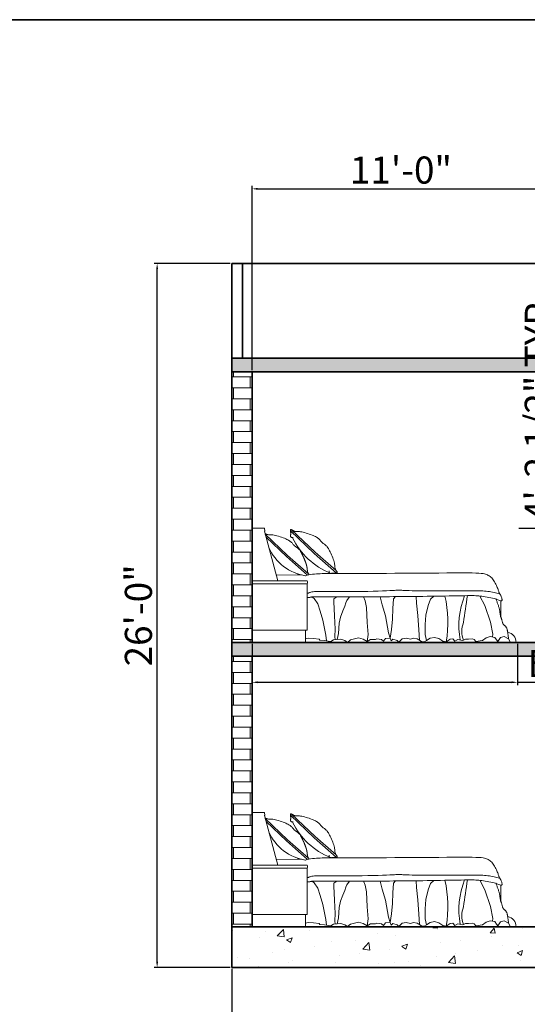
# Model space of a CAD drawing. Units: inches. Extents: x 2142 to 3604, y 1690 to 2981.
# Tile 7 of 9: x 2829 to 3054, y 2545 to 2981. Entities that reach past the tile are written whole.
import ezdxf

# ---------------------------------------------------------------- set-up
doc = ezdxf.new("R2010")
doc.units = ezdxf.units.IN
for name, color, linetype, lineweight in [('A-ANNO-DIMS', 2, 'Continuous', 18), ('A-ANNO-TTLB', 7, 'Continuous', 35), ('A-FLOR-PATT', 8, 'Continuous', 13), ('A-FURN', 8, 'Continuous', 18), ('A-SECT', 7, 'Continuous', 35), ('A-WALL-PATT', 8, 'Continuous', 13)]:
    doc.layers.add(name, color=color, linetype=linetype, lineweight=lineweight)
doc.styles.get("Standard").update_dxf_attribs({"font": 'arial.ttf'})
doc.dimstyles.new('ISO-25', dxfattribs={"dimtxt": 12, "dimasz": 2.5, "dimexe": 1.25, "dimexo": 0.625, "dimtad": 1, "dimdec": 0, "dimlunit": 3, "dimtxsty": 'Standard', "dimcen": 2.5, "dimadec": 0, "dimazin": 0, "dimtfac": 1, "dimtdec": 0, "dimtmove": 0, "dimatfit": 3, "dimfxl": 1, "dimarcsym": 0})

# ---------------------------------------------------------------- blocks, each defined once
blk = doc.blocks.new('A$C08BC4B9A')
for p, q in [((0, 924.5), (0.5, 925)), ((0, 0), (0, 924.5)), ((95, 925), (0.5, 925)), ((101.1, 921.9), (105, 907.4)), ((101.4, 901.2), (208.9, 500)), ((106.6, 881.7), (106.8, 881.6)), ((106.8, 881.6), (109.7, 879.8)), ((109.7, 879.8), (112.8, 878.1)), ((112.8, 878.1), (116.3, 876.5)), ((311.4, 909.3), (311.5, 910.8)), ((311.5, 907.6), (311.4, 909.3)), ((311.5, 910.8), (311.7, 912.1)), ((311.7, 905.6), (311.5, 907.6)), ((311.7, 912.1), (312.1, 913.2)), ((312, 903.5), (311.7, 905.6)), ((502.9, 721.7), (311.9, 904.5)), ((312.3, 901.1), (312, 903.5)), ((312.1, 913.2), (312.7, 914.1)), ((312.6, 898.6), (312.3, 901.1)), ((312.9, 895.9), (312.6, 898.6)), ((312.7, 914.1), (313.6, 914.7)), ((313.1, 892.9), (312.9, 895.9)), ((313.3, 889.8), (313.1, 892.9)), ((313.4, 886.5), (313.3, 889.8)), ((313.3, 875.5), (313.4, 879.4)), ((313.4, 883), (313.4, 886.5)), ((313.4, 879.4), (313.4, 883)), ((313.6, 914.7), (314.7, 915)), ((314.7, 915), (316, 915.1)), ((316, 915.1), (317.6, 914.9)), ((317.6, 914.9), (319.3, 914.5)), ((319.3, 914.5), (321.1, 913.7)), ((511.6, 731.1), (320.5, 913.9)), ((321.1, 913.7), (323.2, 912.6)), ((323.2, 912.6), (325.4, 911.2)), ((325.4, 911.2), (327.8, 909.6)), ((327.8, 909.6), (330.4, 907.8)), ((330.4, 907.8), (333.3, 906.1)), ((333.3, 906.1), (336.4, 904.3)), ((336.4, 904.3), (339.9, 902.7)), ((339.9, 902.7), (343.7, 901.4)), ((343.7, 901.4), (347.9, 900.4)), ((347.9, 900.4), (352.5, 899.8)), ((352.5, 899.8), (357.6, 899.5)), ((357.6, 899.5), (363.2, 899.4)), ((363.2, 899.4), (369.6, 899.2)), ((369.6, 899.2), (376.7, 898.9)), ((376.7, 898.9), (384.6, 898.3)), ((384.6, 898.3), (393.4, 897.3)), ((393.4, 897.3), (403.3, 895.7)), ((403.3, 895.7), (414.2, 893.3)), ((414.2, 893.3), (425.9, 890.4)), ((425.9, 890.4), (438.1, 886.9)), ((438.1, 886.9), (450.5, 883.1)), ((450.5, 883.1), (462.9, 878.9)), ((462.9, 878.9), (474.9, 874.6)), ((288, 704.9), (107.8, 877.3)), ((279.2, 695.5), (114.2, 853.4)), ((116.3, 876.5), (120.1, 875.2)), ((120.1, 875.2), (124.3, 874.2)), ((124.3, 874.2), (128.9, 873.6)), ((128.9, 873.6), (134, 873.3)), ((134, 873.3), (139.6, 873.2)), ((139.6, 873.2), (146, 873)), ((146, 873), (153.1, 872.7)), ((153.1, 872.7), (161, 872.1)), ((161, 872.1), (169.8, 871.1)), ((169.8, 871.1), (179.7, 869.5)), ((179.7, 869.5), (190.6, 867.1)), ((190.6, 867.1), (202.3, 864.2)), ((202.3, 864.2), (214.5, 860.7)), ((214.5, 860.7), (226.9, 856.8)), ((226.9, 856.8), (239.3, 852.7)), ((239.3, 852.7), (251.3, 848.4)), ((251.3, 848.4), (262.7, 844)), ((262.7, 844), (273.2, 839.6)), ((273.2, 839.6), (282.5, 835.5)), ((282.5, 835.5), (290.7, 831.4)), ((290.7, 831.4), (298, 827.4)), ((298, 827.4), (304.4, 823.4)), ((304.4, 823.4), (310.1, 819.5)), ((310.1, 819.5), (315.2, 815.4)), ((312.7, 863.2), (312.8, 867.3)), ((313.1, 859.2), (312.7, 863.2)), ((312.8, 867.3), (313, 871.5)), ((313, 871.5), (313.3, 875.5)), ((314.3, 855.7), (313.1, 859.2)), ((316.7, 852.8), (314.3, 855.7)), ((315.2, 815.4), (319.8, 811.3)), ((320.4, 850.8), (316.7, 852.8)), ((319.8, 811.3), (324.1, 807)), ((325.8, 849.7), (320.4, 850.8)), ((324.1, 807), (328.1, 802.5)), ((333.2, 849.9), (325.8, 849.7)), ((328.1, 802.5), (332, 797.9)), ((332, 797.9), (335.8, 793.2)), ((474.9, 874.6), (486.3, 870.2)), ((486.3, 870.2), (496.8, 865.9)), ((496.8, 865.9), (506.1, 861.7)), ((506.1, 861.7), (514.3, 857.6)), ((514.3, 857.6), (521.6, 853.6)), ((521.6, 853.6), (528, 849.7)), ((528, 849.7), (533.7, 845.7)), ((533.7, 845.7), (538.8, 841.7)), ((538.8, 841.7), (543.4, 837.5)), ((543.4, 837.5), (547.7, 833.2)), ((547.7, 833.2), (551.7, 828.7)), ((551.7, 828.7), (555.6, 824.1)), ((555.6, 824.1), (559.4, 819.4)), ((559.4, 819.4), (563.3, 814.6)), ((563.3, 814.6), (567.7, 810.4)), ((572.2, 806.3), (567.7, 810.4)), ((577.3, 802.8), (572.2, 806.3)), ((582.3, 799.4), (577.3, 802.8)), ((587.2, 795.8), (582.3, 799.4)), ((335.8, 793.2), (339.7, 788.4)), ((339.7, 788.4), (344.1, 784.1)), ((344.2, 784), (344.1, 784.1)), ((344.5, 783.8), (344.2, 784)), ((344.9, 783.4), (344.5, 783.8)), ((345.5, 782.9), (344.9, 783.4)), ((346.1, 782.3), (345.5, 782.9)), ((346.8, 781.7), (346.1, 782.3)), ((347.6, 781.1), (346.8, 781.7)), ((348.3, 780.5), (347.6, 781.1)), ((349.1, 779.9), (348.3, 780.5)), ((349.8, 779.4), (349.1, 779.9)), ((350.5, 778.9), (349.8, 779.4)), ((351.1, 778.4), (350.5, 778.9)), ((351.8, 777.9), (351.1, 778.4)), ((352.4, 777.5), (351.8, 777.9)), ((353.1, 777), (352.4, 777.5)), ((353.7, 776.6), (353.1, 777)), ((354.3, 776.2), (353.7, 776.6)), ((354.9, 775.7), (354.3, 776.2)), ((355.6, 775.3), (354.9, 775.7)), ((356.2, 774.9), (355.6, 775.3)), ((356.8, 774.4), (356.2, 774.9)), ((357.4, 774), (356.8, 774.4)), ((358.1, 773.6), (357.4, 774)), ((358.7, 773.1), (358.1, 773.6)), ((359.3, 772.7), (358.7, 773.1)), ((359.9, 772.3), (359.3, 772.7)), ((360.5, 771.8), (359.9, 772.3)), ((361.2, 771.4), (360.5, 771.8)), ((361.8, 770.9), (361.2, 771.4)), ((362.4, 770.5), (361.8, 770.9)), ((363, 770), (362.4, 770.5)), ((363.6, 769.6), (363, 770)), ((364.2, 769.1), (363.6, 769.6)), ((364.8, 768.7), (364.2, 769.1)), ((365.4, 768.2), (364.8, 768.7)), ((366, 767.8), (365.4, 768.2)), ((366.6, 767.3), (366, 767.8)), ((367.2, 766.8), (366.6, 767.3)), ((367.8, 766.4), (367.2, 766.8)), ((368.3, 765.9), (367.8, 766.4)), ((368.9, 765.4), (368.3, 765.9)), ((369.5, 764.9), (368.9, 765.4)), ((370.1, 764.4), (369.5, 764.9)), ((370.7, 763.9), (370.1, 764.4)), ((371.2, 763.5), (370.7, 763.9)), ((371.8, 763), (371.2, 763.5)), ((372.4, 762.4), (371.8, 763)), ((373, 761.9), (372.4, 762.4)), ((373.5, 761.4), (373, 761.9)), ((374.1, 760.9), (373.5, 761.4)), ((374.7, 760.4), (374.1, 760.9)), ((375.2, 759.8), (374.7, 760.4)), ((375.8, 759.3), (375.2, 759.8)), ((376.3, 758.7), (375.8, 759.3)), ((376.9, 758.2), (376.3, 758.7)), ((377.4, 757.6), (376.9, 758.2)), ((378, 757), (377.4, 757.6)), ((378.6, 756.5), (378, 757)), ((379.2, 755.8), (378.6, 756.5)), ((379.8, 755.2), (379.2, 755.8)), ((380.5, 754.5), (379.8, 755.2)), ((381.3, 753.8), (380.5, 754.5)), ((382.2, 753.1), (381.3, 753.8)), ((383.2, 752.3), (382.2, 753.1)), ((384.2, 751.4), (383.2, 752.3)), ((385.4, 750.5), (384.2, 751.4)), ((386.6, 749.6), (385.4, 750.5)), ((387.8, 748.7), (386.6, 749.6)), ((388.9, 747.8), (387.8, 748.7)), ((389.9, 746.9), (388.9, 747.8)), ((390.8, 746), (389.9, 746.9)), ((391.4, 745.3), (390.8, 746)), ((391.9, 744.6), (391.4, 745.3)), ((392.1, 744), (391.9, 744.6)), ((392, 741.9), (392.1, 742.4)), ((392, 741.3), (392, 741.9)), ((392, 740.8), (392, 741.3)), ((392.1, 740.1), (392, 740.8)), ((392.2, 743.4), (392.1, 744)), ((392.1, 742.4), (392.2, 742.9)), ((392.4, 739.4), (392.1, 740.1)), ((392.2, 742.9), (392.2, 743.4)), ((392.7, 738.6), (392.4, 739.4)), ((393.1, 737.8), (392.7, 738.6)), ((393.6, 737), (393.1, 737.8)), ((394.1, 736.1), (393.6, 737)), ((394.7, 735.2), (394.1, 736.1)), ((395.2, 734.3), (394.7, 735.2)), ((395.8, 733.4), (395.2, 734.3)), ((396.4, 732.4), (395.8, 733.4)), ((397, 731.5), (396.4, 732.4)), ((397.6, 730.5), (397, 731.5)), ((398.2, 729.5), (397.6, 730.5)), ((398.7, 728.5), (398.2, 729.5)), ((399.3, 727.4), (398.7, 728.5)), ((399.9, 726.4), (399.3, 727.4)), ((400.5, 725.3), (399.9, 726.4)), ((401.1, 724.3), (400.5, 725.3)), ((401.7, 723.2), (401.1, 724.3)), ((402.4, 722), (401.7, 723.2)), ((403, 720.9), (402.4, 722)), ((403.6, 719.8), (403, 720.9)), ((404.2, 718.6), (403.6, 719.8)), ((404.8, 717.4), (404.2, 718.6)), ((685.7, 562.3), (502.9, 721.7)), ((681.3, 583.2), (511.6, 731.1)), ((592, 792.2), (587.2, 795.8)), ((596.6, 788.2), (592, 792.2)), ((601.1, 783.9), (596.6, 788.2)), ((605.5, 779.1), (601.1, 783.9)), ((609.9, 773.7), (605.5, 779.1)), ((614.3, 767.6), (609.9, 773.7)), ((618.8, 760.7), (614.3, 767.6)), ((623.5, 752.8), (618.8, 760.7)), ((628.4, 743.8), (623.5, 752.8)), ((633.5, 733.7), (628.4, 743.8)), ((638.7, 722.7), (633.5, 733.7)), ((643.9, 711), (638.7, 722.7)), ((450.1, 546.6), (279.2, 695.5)), ((457.7, 557), (288, 704.9)), ((405.4, 716.2), (404.8, 717.4)), ((406.1, 715), (405.4, 716.2)), ((406.7, 713.8), (406.1, 715)), ((407.3, 712.5), (406.7, 713.8)), ((408, 711.2), (407.3, 712.5)), ((408.6, 710), (408, 711.2)), ((409.3, 708.7), (408.6, 710)), ((409.9, 707.3), (409.3, 708.7)), ((410.6, 706), (409.9, 707.3)), ((411.2, 704.7), (410.6, 706)), ((411.9, 703.3), (411.2, 704.7)), ((412.5, 701.9), (411.9, 703.3)), ((413.2, 700.6), (412.5, 701.9)), ((413.8, 699.2), (413.2, 700.6)), ((414.5, 697.8), (413.8, 699.2)), ((415.1, 696.4), (414.5, 697.8)), ((415.8, 694.9), (415.1, 696.4)), ((416.4, 693.5), (415.8, 694.9)), ((417.1, 692.1), (416.4, 693.5)), ((417.7, 690.6), (417.1, 692.1)), ((418.4, 689.2), (417.7, 690.6)), ((419, 687.7), (418.4, 689.2)), ((419.7, 686.2), (419, 687.7)), ((420.3, 684.7), (419.7, 686.2)), ((421, 683.3), (420.3, 684.7)), ((421.6, 681.8), (421, 683.3)), ((422.2, 680.3), (421.6, 681.8)), ((422.9, 678.8), (422.2, 680.3)), ((423.5, 677.3), (422.9, 678.8)), ((424.1, 675.8), (423.5, 677.3)), ((424.7, 674.3), (424.1, 675.8)), ((425.4, 672.8), (424.7, 674.3)), ((426, 671.3), (425.4, 672.8)), ((426.6, 669.7), (426, 671.3)), ((427.2, 668.2), (426.6, 669.7)), ((427.8, 666.7), (427.2, 668.2)), ((428.4, 665.2), (427.8, 666.7)), ((429, 663.7), (428.4, 665.2)), ((429.6, 662.2), (429, 663.7)), ((430.1, 660.7), (429.6, 662.2)), ((430.7, 659.2), (430.1, 660.7)), ((431.3, 657.7), (430.7, 659.2)), ((431.8, 656.2), (431.3, 657.7)), ((432.4, 654.7), (431.8, 656.2)), ((432.9, 653.2), (432.4, 654.7)), ((433.4, 651.8), (432.9, 653.2)), ((434, 650.3), (433.4, 651.8)), ((434.5, 648.8), (434, 650.3)), ((435, 647.4), (434.5, 648.8)), ((435.5, 645.9), (435, 647.4)), ((436, 644.5), (435.5, 645.9)), ((436.5, 643.1), (436, 644.5)), ((436.9, 641.7), (436.5, 643.1)), ((437.4, 640.2), (436.9, 641.7)), ((437.9, 638.8), (437.4, 640.2)), ((438.3, 637.5), (437.9, 638.8)), ((649, 699), (643.9, 711)), ((653.8, 686.9), (649, 699)), ((658.2, 675), (653.8, 686.9)), ((662, 663.6), (658.2, 675)), ((665.2, 652.9), (662, 663.6)), ((667.5, 643.2), (665.2, 652.9)), ((669.2, 634.4), (667.5, 643.2)), ((438.7, 636.1), (438.3, 637.5)), ((439.1, 634.7), (438.7, 636.1)), ((439.6, 633.4), (439.1, 634.7)), ((440, 632), (439.6, 633.4)), ((440.3, 630.7), (440, 632)), ((440.7, 629.4), (440.3, 630.7)), ((441.1, 628.1), (440.7, 629.4)), ((441.4, 626.8), (441.1, 628.1)), ((441.8, 625.5), (441.4, 626.8)), ((442.1, 624.3), (441.8, 625.5)), ((442.4, 623.1), (442.1, 624.3)), ((442.7, 621.8), (442.4, 623.1)), ((443, 620.6), (442.7, 621.8)), ((443.3, 619.4), (443, 620.6)), ((443.6, 618.3), (443.3, 619.4)), ((443.8, 617.1), (443.6, 618.3)), ((444.1, 616), (443.8, 617.1)), ((444.3, 614.8), (444.1, 616)), ((444.5, 613.7), (444.3, 614.8)), ((444.7, 612.6), (444.5, 613.7)), ((445, 611.5), (444.7, 612.6)), ((445.2, 610.5), (445, 611.5)), ((445.4, 609.4), (445.2, 610.5)), ((445.5, 608.4), (445.4, 609.4)), ((445.7, 607.3), (445.5, 608.4)), ((445.9, 606.3), (445.7, 607.3)), ((446, 605.3), (445.9, 606.3)), ((446.2, 604.3), (446, 605.3)), ((446.4, 603.3), (446.2, 604.3)), ((446.5, 602.4), (446.4, 603.3)), ((446.6, 601.4), (446.5, 602.4)), ((446.8, 600.5), (446.6, 601.4)), ((446.9, 599.6), (446.8, 600.5)), ((447, 598.6), (446.9, 599.6)), ((447.1, 597.7), (447, 598.6)), ((447.2, 596.9), (447.1, 597.7)), ((447.3, 596), (447.2, 596.9)), ((447.4, 595.1), (447.3, 596)), ((447.5, 594.3), (447.4, 595.1)), ((447.6, 593.4), (447.5, 594.3)), ((447.7, 592.6), (447.6, 593.4)), ((447.8, 591.8), (447.7, 592.6)), ((447.9, 591), (447.8, 591.8)), ((448, 590.2), (447.9, 591)), ((448, 589.4), (448, 590.2)), ((448.1, 588.6), (448, 589.4)), ((448.2, 587.9), (448.1, 588.6)), ((448.3, 587.1), (448.2, 587.9)), ((448.3, 586.4), (448.3, 587.1)), ((448.4, 585.6), (448.3, 586.4)), ((448.5, 584.9), (448.4, 585.6)), ((448.6, 584.2), (448.5, 584.9)), ((448.6, 583.5), (448.6, 584.2)), ((448.7, 582.8), (448.6, 583.5)), ((448.8, 582.1), (448.7, 582.8)), ((448.9, 581.4), (448.8, 582.1)), ((448.9, 580.8), (448.9, 581.4)), ((449, 580.1), (448.9, 580.8)), ((449.1, 579.5), (449, 580.1)), ((449.2, 578.8), (449.1, 579.5)), ((449.3, 578.2), (449.2, 578.8)), ((449.4, 577.6), (449.3, 578.2)), ((449.5, 577), (449.4, 577.6)), ((449.6, 576.4), (449.5, 577)), ((449.7, 575.8), (449.6, 576.4)), ((449.8, 575.2), (449.7, 575.8)), ((449.9, 574.6), (449.8, 575.2)), ((450, 574), (449.9, 574.6)), ((450.1, 573.5), (450, 574)), ((450.3, 572.9), (450.1, 573.5)), ((450.4, 572.4), (450.3, 572.9)), ((450.5, 571.8), (450.4, 572.4)), ((450.7, 571.3), (450.5, 571.8)), ((450.8, 570.8), (450.7, 571.3)), ((451, 570.2), (450.8, 570.8)), ((451.1, 569.7), (451, 570.2)), ((451.3, 569.2), (451.1, 569.7)), ((451.5, 568.7), (451.3, 569.2)), ((451.6, 568.2), (451.5, 568.7)), ((451.8, 567.7), (451.6, 568.2)), ((452, 567.2), (451.8, 567.7)), ((452.2, 566.8), (452, 567.2)), ((452.4, 566.3), (452.2, 566.8)), ((452.6, 565.8), (452.4, 566.3)), ((452.8, 565.4), (452.6, 565.8)), ((453, 564.9), (452.8, 565.4)), ((453.2, 564.5), (453, 564.9)), ((453.4, 564), (453.2, 564.5)), ((453.6, 563.6), (453.4, 564)), ((453.8, 563.1), (453.6, 563.6)), ((454.1, 562.7), (453.8, 563.1)), ((454.3, 562.3), (454.1, 562.7)), ((454.5, 561.9), (454.3, 562.3)), ((454.8, 561.5), (454.5, 561.9)), ((455, 561.1), (454.8, 561.5)), ((455.2, 560.7), (455, 561.1)), ((455.5, 560.3), (455.2, 560.7)), ((455.7, 559.9), (455.5, 560.3)), ((456, 559.5), (455.7, 559.9)), ((456.2, 559.1), (456, 559.5)), ((456.4, 558.8), (456.2, 559.1)), ((456.7, 558.4), (456.4, 558.8)), ((586, 558.6), (569.7, 558.1)), ((603.2, 559), (586, 558.6)), ((621.8, 559.3), (603.2, 559)), ((642.6, 559.5), (621.8, 559.3)), ((624.8, 579.5), (625.2, 572.1)), ((625.2, 572.1), (626.6, 566.8)), ((626.6, 566.8), (629, 563.3)), ((629, 563.3), (632, 561.2)), ((632, 561.2), (635.6, 560.2)), ((635.6, 560.2), (639.6, 560.1)), ((639.6, 560.1), (643.7, 560.5)), ((666.5, 559.6), (642.6, 559.5)), ((643.7, 560.5), (647.9, 561)), ((647.9, 561), (651.9, 561.6)), ((651.9, 561.6), (655.7, 562)), ((655.7, 562), (659.3, 562.3)), ((659.3, 562.3), (662.8, 562.5)), ((662.8, 562.5), (666.1, 562.7)), ((666.1, 562.7), (669.2, 562.7)), ((693.9, 559.6), (666.5, 559.6)), ((670.4, 626.6), (669.2, 634.4)), ((669.2, 562.7), (672.2, 562.7)), ((671.3, 619.5), (670.4, 626.6)), ((671.9, 613.2), (671.3, 619.5)), ((672.5, 607.6), (671.9, 613.2)), ((672.2, 562.7), (674.9, 562.7)), ((673.1, 602.5), (672.5, 607.6)), ((674.1, 598), (673.1, 602.5)), ((675.4, 593.9), (674.1, 598)), ((674.9, 562.7), (677.5, 562.6)), ((677, 590.2), (675.4, 593.9)), ((678.8, 586.8), (677, 590.2)), ((677.5, 562.6), (679.8, 562.4)), ((680.8, 583.8), (678.8, 586.8)), ((679.8, 562.4), (682, 562.3)), ((682.8, 581.1), (680.8, 583.8)), ((682, 562.3), (683.9, 562.3)), ((684.7, 578.6), (682.8, 581.1)), ((683.9, 562.3), (685.7, 562.3)), ((686.5, 576.4), (684.7, 578.6)), ((685.7, 562.3), (687.2, 562.4)), ((688.1, 574.3), (686.5, 576.4)), ((687.2, 562.4), (688.5, 562.7)), ((689.3, 572.3), (688.1, 574.3)), ((688.5, 562.7), (689.5, 563.2)), ((690.2, 570.5), (689.3, 572.3)), ((689.5, 563.2), (690.3, 563.9)), ((690.8, 568.8), (690.2, 570.5)), ((690.3, 563.9), (690.9, 564.9)), ((691.1, 567.3), (690.8, 568.8)), ((690.9, 564.9), (691.1, 566)), ((691.1, 566), (691.1, 567.3)), ((725.8, 559.7), (693.9, 559.6)), ((762.8, 559.7), (725.8, 559.7)), ((805.4, 559.7), (762.8, 559.7)), ((853.4, 559.7), (805.4, 559.7)), ((906.2, 559.7), (853.4, 559.7)), ((963.4, 559.8), (906.2, 559.7)), ((1024.6, 559.9), (963.4, 559.8)), ((1089.2, 560.1), (1024.6, 559.9)), ((1156.7, 560.4), (1089.2, 560.1)), ((1226.8, 560.7), (1156.7, 560.4)), ((1298.7, 561.1), (1226.8, 560.7)), ((1371.2, 561.6), (1298.7, 561.1)), ((1443.1, 562.1), (1371.2, 561.6)), ((1512.8, 562.6), (1443.1, 562.1)), ((1579.1, 563), (1512.8, 562.6)), ((1640.5, 563.3), (1579.1, 563)), ((1695.8, 563.4), (1640.5, 563.3)), ((1743.5, 563.3), (1695.8, 563.4)), ((1782.8, 563), (1743.5, 563.3)), ((1814.2, 562.4), (1782.8, 563)), ((1838.9, 561.5), (1814.2, 562.4)), ((1858, 560.2), (1838.9, 561.5)), ((1872.6, 558.6), (1858, 560.2)), ((1883.7, 556.6), (1872.6, 558.6)), ((445.9, 500), (0, 500)), ((366.1, 546.8), (196.6, 546.1)), ((400.7, 547.5), (366.1, 546.8)), ((420, 543.6), (400.7, 547.5)), ((431.7, 540.1), (420, 543.6)), ((439.4, 542.5), (431.7, 540.1)), ((445.4, 545.7), (439.4, 542.5)), ((460.2, 548.4), (445.4, 545.7)), ((456.9, 558), (456.7, 558.4)), ((457.2, 557.7), (456.9, 558)), ((457.4, 557.3), (457.2, 557.7)), ((457.7, 557), (457.4, 557.3)), ((457.9, 556.6), (457.7, 557)), ((458.2, 556.3), (457.9, 556.6)), ((458.4, 555.9), (458.2, 556.3)), ((458.7, 555.6), (458.4, 555.9)), ((458.9, 555.3), (458.7, 555.6)), ((459.2, 554.9), (458.9, 555.3)), ((459.4, 554.6), (459.2, 554.9)), ((459.7, 554.3), (459.4, 554.6)), ((459.9, 554), (459.7, 554.3)), ((460.2, 553.6), (459.9, 554)), ((460.4, 553.3), (460.2, 553.6)), ((475.2, 550.7), (460.2, 548.4)), ((460.7, 553), (460.4, 553.3)), ((461, 552.6), (460.7, 553)), ((461.3, 552.3), (461, 552.6)), ((461.6, 551.9), (461.3, 552.3)), ((461.9, 551.5), (461.6, 551.9)), ((462.2, 551.1), (461.9, 551.5)), ((462.5, 550.7), (462.2, 551.1)), ((462.8, 550.3), (462.5, 550.7)), ((463.2, 549.8), (462.8, 550.3)), ((463.5, 549.4), (463.2, 549.8)), ((463.8, 548.9), (463.5, 549.4)), ((490.5, 552.6), (475.2, 550.7)), ((506, 554.2), (490.5, 552.6)), ((521.7, 555.5), (506, 554.2)), ((537.6, 556.6), (521.7, 555.5)), ((553.6, 557.4), (537.6, 556.6)), ((569.7, 558.1), (553.6, 557.4)), ((1892.6, 554.2), (1883.7, 556.6)), ((1900.3, 551.3), (1892.6, 554.2)), ((1907.7, 547.9), (1900.3, 551.3)), ((1915, 544), (1907.7, 547.9)), ((1922.1, 539.6), (1915, 544)), ((1929, 534.5), (1922.1, 539.6)), ((1935.8, 528.9), (1929, 534.5)), ((1942.3, 522.6), (1935.8, 528.9)), ((1948.6, 515.6), (1942.3, 522.6)), ((1954.6, 508), (1948.6, 515.6)), ((1960.4, 499.6), (1954.6, 508)), ((1965.8, 490.7), (1960.4, 499.6)), ((1970.9, 481.5), (1965.8, 490.7)), ((1975.6, 472.1), (1970.9, 481.5)), ((445.9, 475), (0, 475)), ((445.9, 475), (445.9, 100)), ((449.1, 398.3), (453.4, 399.2)), ((453.4, 399.2), (457.6, 400.4)), ((457.6, 400.4), (461.8, 402)), ((461.8, 402), (466.2, 403.7)), ((466.2, 403.7), (471.3, 405.6)), ((471.3, 405.6), (477.6, 407.5)), ((477.6, 407.5), (485.4, 409.4)), ((485.4, 409.4), (495.3, 411.1)), ((495.3, 411.1), (507.7, 412.5)), ((507.7, 412.5), (523, 413.5)), ((523, 413.5), (541.5, 414)), ((541.5, 414), (563.2, 414.2)), ((563.2, 414.2), (588.2, 414.1)), ((588.2, 414.1), (616.4, 413.7)), ((616.4, 413.7), (647.7, 413.3)), ((647.7, 413.3), (682, 412.9)), ((682, 412.9), (719.4, 412.6)), ((719.4, 412.6), (759.7, 412.4)), ((759.7, 412.4), (802.6, 412.6)), ((802.6, 412.6), (847.4, 413)), ((847.4, 413), (892.8, 413.6)), ((892.8, 413.6), (937.8, 414.4)), ((937.8, 414.4), (981.1, 415.3)), ((981.1, 415.3), (1021.7, 416.4)), ((1021.7, 416.4), (1058.6, 417.5)), ((1058.6, 417.5), (1090.4, 418.7)), ((1090.4, 418.7), (1116.5, 419.9)), ((1116.5, 419.9), (1137.2, 421)), ((1137.2, 421), (1153.4, 422.1)), ((1153.4, 422.1), (1165.7, 423)), ((1165.7, 423), (1174.9, 423.8)), ((1174.9, 423.8), (1181.7, 424.4)), ((1181.7, 424.4), (1186.9, 424.8)), ((1186.9, 424.8), (1191.2, 425)), ((1191.2, 425), (1195.4, 424.8)), ((1195.4, 424.8), (1200, 424.5)), ((1200, 424.5), (1205.8, 423.9)), ((1205.8, 423.9), (1213.3, 423.2)), ((1213.3, 423.2), (1223.1, 422.4)), ((1223.1, 422.4), (1236, 421.7)), ((1236, 421.7), (1252.5, 420.9)), ((1252.5, 420.9), (1273.3, 420.3)), ((1273.3, 420.3), (1298.7, 419.7)), ((1298.7, 419.7), (1328.3, 419.4)), ((1328.3, 419.4), (1361.1, 419.1)), ((1361.1, 419.1), (1396.4, 418.9)), ((1396.4, 418.9), (1433.4, 418.8)), ((1433.4, 418.8), (1471.3, 418.7)), ((1471.3, 418.7), (1509.3, 418.7)), ((1509.3, 418.7), (1546.6, 418.7)), ((1546.6, 418.7), (1582.4, 418.7)), ((1582.4, 418.7), (1616.7, 418.7)), ((1616.7, 418.7), (1649.3, 418.7)), ((1649.3, 418.7), (1680.1, 418.7)), ((1680.1, 418.7), (1709, 418.7)), ((1709, 418.7), (1736, 418.7)), ((1736, 418.7), (1760.9, 418.7)), ((1760.9, 418.7), (1783.8, 418.7)), ((1783.8, 418.7), (1804.5, 418.7)), ((1804.5, 418.7), (1823.2, 418.6)), ((1823.2, 418.6), (1840.3, 418.5)), ((1840.3, 418.5), (1856.1, 418.1)), ((1856.1, 418.1), (1870.7, 417.6)), ((1870.7, 417.6), (1884.5, 416.7)), ((1884.5, 416.7), (1897.8, 415.6)), ((1897.8, 415.6), (1910.8, 414)), ((1910.8, 414), (1923.7, 412)), ((1923.7, 412), (1936.5, 409.7)), ((1936.5, 409.7), (1949.1, 407.1)), ((1949.1, 407.1), (1961.3, 404.4)), ((1961.3, 404.4), (1973.1, 401.6)), ((1973.1, 401.6), (1984.4, 398.8)), ((1980, 462.7), (1975.6, 472.1)), ((1984, 453.6), (1980, 462.7)), ((1987.5, 445), (1984, 453.6)), ((1990.7, 437), (1987.5, 445)), ((1993.4, 429.7), (1990.7, 437)), ((1995.8, 423.3), (1993.4, 429.7)), ((1997.8, 417.5), (1995.8, 423.3)), ((1999.6, 412.4), (1997.8, 417.5)), ((2001.3, 407.8), (1999.6, 412.4)), ((2002.8, 403.7), (2001.3, 407.8)), ((2004.3, 400.1), (2002.8, 403.7)), ((2005.8, 396.8), (2004.3, 400.1)), ((445.9, 397.8), (449.1, 398.3)), ((445.9, 362), (481.5, 369.7)), ((445.9, 362.5), (450.4, 363.2)), ((450.4, 363.2), (457.2, 364.1)), ((457.2, 364.1), (463.4, 364.9)), ((463.4, 364.9), (468.9, 365.7)), ((468.9, 365.7), (473.6, 366.4)), ((473.6, 366.4), (477.6, 367.1)), ((477.6, 367.1), (481.1, 367.7)), ((481.1, 367.7), (484.4, 368.3)), ((484.4, 368.3), (488, 368.8)), ((504.7, 356.4), (486.2, 368.5)), ((488, 368.8), (492.3, 369.2)), ((492.3, 369.2), (497.5, 369.6)), ((497.5, 369.6), (504.1, 369.9)), ((504.1, 369.9), (512.5, 370.1)), ((534.3, 312.8), (504.7, 356.4)), ((512.5, 370.1), (522.9, 370.3)), ((522.9, 370.3), (535.3, 370.3)), ((535.3, 370.3), (549.5, 370.3)), ((549.5, 370.3), (565.4, 370.3)), ((565.4, 370.3), (582.8, 370.2)), ((582.8, 370.2), (601.6, 370.2)), ((601.6, 370.2), (621.6, 370.1)), ((621.6, 370.1), (642.7, 370.1)), ((642.7, 370.1), (664.7, 370.1)), ((663.6, 354.7), (661.8, 330.2)), ((661.8, 330.2), (668.8, 215.1)), ((687.3, 370.2), (663.6, 354.7)), ((664.7, 370.1), (687.3, 370.2)), ((687.3, 370.2), (710.4, 370.3)), ((710.4, 370.3), (733.4, 370.4)), ((733.4, 370.4), (756.3, 370.4)), ((750.9, 293.6), (759.6, 321.5)), ((756.3, 370.4), (778.7, 370.5)), ((759.6, 321.5), (768.3, 339)), ((768.3, 339), (789.4, 370.5)), ((778.7, 370.5), (800.2, 370.6)), ((800.2, 370.6), (820.7, 370.6)), ((820.7, 370.6), (840, 370.6)), ((840, 370.6), (858.3, 370.5)), ((858.3, 370.5), (876.2, 370.4)), ((876.2, 370.4), (894, 370.4)), ((894, 370.4), (912.3, 370.3)), ((916.7, 337.2), (903.2, 370.3)), ((912.3, 370.3), (931.5, 370.2)), ((927.2, 283.1), (916.7, 337.2)), ((931.5, 370.2), (952, 370.2)), ((952, 370.2), (974.3, 370.2)), ((974.3, 370.2), (998.7, 370.3)), ((998.7, 370.3), (1025.1, 370.4)), ((1025.1, 370.4), (1053.2, 370.6)), ((1054.7, 305.8), (1039.1, 370.5)), ((1053.2, 370.6), (1082.9, 370.8)), ((1082.9, 370.8), (1113.8, 371)), ((1113.8, 371), (1145.8, 371.3)), ((1145.5, 354.7), (1140.2, 274.4)), ((1162.2, 371.4), (1145.5, 354.7)), ((1145.8, 371.3), (1178.6, 371.6)), ((1178.6, 371.6), (1212, 371.9)), ((1212, 371.9), (1245.7, 372.2)), ((1245.7, 372.2), (1279.8, 372.6)), ((1279.8, 372.6), (1314.1, 373)), ((1314.1, 373), (1348.8, 373.4)), ((1332.3, 318), (1331.5, 373.2)), ((1348.8, 373.4), (1383.8, 373.8)), ((1383.8, 373.8), (1419.1, 374.3)), ((1419.1, 374.3), (1454.7, 374.8)), ((1428.3, 300.6), (1445.8, 351.2)), ((1445.8, 351.2), (1472.7, 375.1)), ((1454.7, 374.8), (1490.6, 375.4)), ((1490.6, 375.4), (1526.8, 376)), ((1526.8, 376), (1562.7, 376.6)), ((1562.7, 376.6), (1597.9, 377.2)), ((1597.9, 377.2), (1632, 377.8)), ((1632, 377.8), (1664.4, 378.4)), ((1664.4, 378.4), (1694.6, 378.9)), ((1694.6, 378.9), (1722.2, 379.3)), ((1722.2, 379.3), (1746.7, 379.5)), ((1746.7, 379.5), (1767.7, 379.7)), ((1767.7, 379.7), (1785.7, 379.6)), ((1785.7, 379.6), (1801.2, 379.4)), ((1801.2, 379.4), (1814.9, 378.9)), ((1814.9, 378.9), (1827.4, 378.2)), ((1827.4, 378.2), (1839.2, 377.2)), ((1839.2, 377.2), (1850.9, 375.9)), ((1845.1, 376.6), (1887, 298.9)), ((1850.9, 375.9), (1863.2, 374.3)), ((1863.2, 374.3), (1876.4, 372.4)), ((1876.4, 372.4), (1890.5, 370.2)), ((1890.5, 370.2), (1905, 367.7)), ((1905, 367.7), (1919.7, 364.9)), ((1919.7, 364.9), (1934.2, 362)), ((1934.2, 362), (1948.2, 358.9)), ((1948.2, 358.9), (1961.4, 355.7)), ((1961.4, 355.7), (1973.5, 352.4)), ((1973.5, 352.4), (1984.1, 349.1)), ((1977.1, 352.6), (1976.8, 353.5)), ((1978, 350), (1977.1, 352.6)), ((1979.4, 346.1), (1978, 350)), ((1981.2, 341.1), (1979.4, 346.1)), ((1983.2, 335.3), (1981.2, 341.1)), ((1985.5, 329), (1983.2, 335.3)), ((1984.1, 349.1), (1993.3, 345.9)), ((1984.4, 398.8), (1995, 396.1)), ((1987.8, 322.5), (1985.5, 329)), ((1990.1, 316.1), (1987.8, 322.5)), ((1993.3, 345.9), (2001.3, 342.9)), ((1995, 396.1), (2004.8, 393.6)), ((2001.3, 342.9), (2007.9, 340.5)), ((2007.5, 393.8), (2005.8, 396.8)), ((2009.2, 390.9), (2007.5, 393.8)), ((2007.9, 340.5), (2013.4, 338.6)), ((2010.9, 388.2), (2009.2, 390.9)), ((2012.7, 385.4), (2010.9, 388.2)), ((2014.5, 382.5), (2012.7, 385.4)), ((2013.4, 338.6), (2017.8, 337.5)), ((2016.4, 379.3), (2014.5, 382.5)), ((2015, 211.3), (2015, 338.2)), ((2018.2, 375.7), (2016.4, 379.3)), ((2017.8, 337.5), (2021.2, 337.3)), ((2020, 371.7), (2018.2, 375.7)), ((2021.7, 367.2), (2020, 371.7)), ((2021.2, 337.3), (2023.6, 338.3)), ((2023.2, 362.2), (2021.7, 367.2)), ((2024.6, 357.2), (2023.2, 362.2)), ((2023.6, 338.3), (2025.2, 340.5)), ((2025.5, 352.3), (2024.6, 357.2)), ((2025.2, 340.5), (2025.9, 343.7)), ((2026, 347.7), (2025.5, 352.3)), ((2025.9, 343.7), (2026, 347.7)), ((551.8, 253.5), (534.3, 312.8)), ((572.8, 180.2), (551.8, 253.5)), ((717.7, 206.4), (736.9, 257)), ((736.9, 257), (750.9, 293.6)), ((934.2, 161), (927.2, 283.1)), ((1082.6, 216.8), (1054.7, 305.8)), ((1140.2, 274.4), (1138.5, 188.9)), ((1342.8, 218.6), (1332.3, 318)), ((1409.1, 220.3), (1428.3, 300.6)), ((1887, 298.9), (1932.4, 164.5)), ((1992.3, 309.9), (1990.1, 316.1)), ((1994.4, 304), (1992.3, 309.9)), ((1996.4, 298.3), (1994.4, 304)), ((1998.2, 292.7), (1996.4, 298.3)), ((2000, 287.1), (1998.2, 292.7)), ((2001.6, 281.3), (2000, 287.1)), ((2003.1, 275.4), (2001.6, 281.3)), ((2004.5, 269.2), (2003.1, 275.4)), ((2005.8, 262.6), (2004.5, 269.2)), ((2006.9, 255.8), (2005.8, 262.6)), ((2008, 248.9), (2006.9, 255.8)), ((2009, 242.1), (2008, 248.9)), ((2010, 235.6), (2009, 242.1)), ((597.2, 59.8), (572.8, 180.2)), ((668.8, 215.1), (674, 106.9)), ((707.2, 155.8), (717.7, 206.4)), ((941.2, 65.1), (934.2, 161)), ((1105.3, 77.3), (1082.6, 216.8)), ((1138.5, 188.9), (1131.5, 105.2)), ((1353.2, 103.4), (1342.8, 218.6)), ((1403.9, 145.3), (1409.1, 220.3)), ((1932.4, 164.5), (1951.6, 66.8)), ((2011, 229.5), (2010, 235.6)), ((2011.9, 223.9), (2011, 229.5)), ((2012.9, 219), (2011.9, 223.9)), ((2013.9, 215), (2012.9, 219)), ((2014.9, 211.6), (2013.9, 215)), ((2015.9, 208.7), (2014.9, 211.6)), ((2017, 206), (2015.9, 208.7)), ((2018.1, 203.5), (2017, 206)), ((2019.2, 200.8), (2018.1, 203.5)), ((2020.3, 197.8), (2019.2, 200.8)), ((2021.4, 194.3), (2020.3, 197.8)), ((2022.5, 190.2), (2021.4, 194.3)), ((2023.7, 185.5), (2022.5, 190.2)), ((2024.9, 180.4), (2023.7, 185.5)), ((2026.1, 175.1), (2024.9, 180.4)), ((2027.4, 169.8), (2026.1, 175.1)), ((2028.9, 164.7), (2027.4, 169.8)), ((2030.5, 159.8), (2028.9, 164.7)), ((2032.2, 155.5), (2030.5, 159.8)), ((445.9, 100), (0, 100)), ((433.9, 100), (433.9, 0)), ((674, 106.9), (672.3, 47.6)), ((702, 72), (707.2, 155.8)), ((1131.5, 105.2), (1119, 34)), ((1356.3, 18.2), (1353.2, 103.4)), ((1403.9, 65.1), (1403.9, 145.3)), ((2034.1, 151.8), (2032.2, 155.5)), ((2036.1, 148.6), (2034.1, 151.8)), ((2038.3, 145.9), (2036.1, 148.6)), ((2040.5, 143.6), (2038.3, 145.9)), ((2042.8, 141.5), (2040.5, 143.6)), ((2045, 139.6), (2042.8, 141.5)), ((2047.3, 137.8), (2045, 139.6)), ((2049.5, 136), (2047.3, 137.8)), ((2051.6, 134.1), (2049.5, 136)), ((2053.6, 132), (2051.6, 134.1)), ((2055.6, 129.7), (2053.6, 132)), ((2057.4, 127.3), (2055.6, 129.7)), ((2059.1, 124.7), (2057.4, 127.3)), ((2060.8, 121.9), (2059.1, 124.7)), ((2062.3, 118.9), (2060.8, 121.9)), ((2063.8, 115.6), (2062.3, 118.9)), ((2065.1, 112), (2063.8, 115.6)), ((2066.4, 108.3), (2065.1, 112)), ((2067.5, 104.3), (2066.4, 108.3)), ((2068.6, 100.2), (2067.5, 104.3)), ((2069.5, 95.9), (2068.6, 100.2)), ((2070.4, 91.5), (2069.5, 95.9)), ((2071.2, 87), (2070.4, 91.5)), ((2072, 82.5), (2071.2, 87)), ((2072.6, 77.9), (2072, 82.5)), ((0, 0), (2150.5, 0)), ((433.9, 29.5), (455.7, 35.6)), ((455.7, 35.6), (497.9, 32.5)), ((497.9, 32.5), (543.3, 26.2)), ((543.3, 26.2), (549.6, 18.4)), ((549.6, 18.4), (587.1, 16.9)), ((587.1, 16.9), (618.4, 10.6)), ((602.8, 13.7), (597.2, 59.8)), ((618.4, 10.6), (638.7, 9)), ((638.7, 9), (660.6, 21.5)), ((660.6, 21.5), (720.1, 26.2)), ((672.3, 47.6), (674.3, 22.6)), ((690.4, 23.9), (702, 72)), ((720.1, 26.2), (752.9, 16.9)), ((752.9, 16.9), (773.3, 1.2)), ((773.3, 1.2), (798.3, 21.5)), ((798.3, 21.5), (864, 37.2)), ((864, 37.2), (900, 27.8)), ((900, 27.8), (932.8, 7.5)), ((932.8, 7.5), (941.2, 65.1)), ((932.8, 7.5), (961, 24.7)), ((961, 24.7), (1000.1, 23.1)), ((1000.1, 23.1), (1011.1, 29.4)), ((1011.1, 29.4), (1048.6, 23.1)), ((1048.6, 23.1), (1064.3, 10.6)), ((1064.3, 10.6), (1081.5, 32.5)), ((1081.5, 32.5), (1119, 34)), ((1119, 34), (1105.3, 77.3)), ((1119, 34), (1128.4, 12.2)), ((1128.4, 12.2), (1142.5, 26.2)), ((1142.5, 26.2), (1175.3, 16.9)), ((1175.3, 16.9), (1191, 2.8)), ((1191, 2.8), (1217.6, 29.4)), ((1217.6, 29.4), (1250.4, 35.6)), ((1250.4, 35.6), (1283.3, 26.2)), ((1283.3, 26.2), (1307.8, 35.4)), ((1307.8, 35.4), (1339.1, 29.2)), ((1339.1, 29.2), (1373.5, 7.3)), ((1373.5, 7.3), (1393.8, 5.7)), ((1393.8, 5.7), (1414.2, 16.7)), ((1414.2, 16.7), (1403.9, 65.1)), ((1414.2, 16.7), (1443.9, 33.9)), ((1443.9, 33.9), (1478.3, 41.7)), ((1478.3, 41.7), (1514.3, 32.3)), ((1514.3, 32.3), (1547.2, 10.4)), ((1547.2, 10.4), (1573.7, 5.7)), ((1573.7, 5.7), (1606.6, 26.1)), ((1606.6, 26.1), (1628.5, 29.2)), ((1628.5, 29.2), (1642.6, 10.4)), ((1642.6, 10.4), (1667.6, 24.5)), ((1667.6, 24.5), (1705.2, 16.7)), ((1705.2, 16.7), (1714.5, 18.2)), ((1714.5, 18.2), (1730.2, 27.6)), ((1730.2, 27.6), (1745.8, 27.6)), ((1745.8, 27.6), (1753.7, 27.6)), ((1753.7, 27.6), (1786.5, 30.7)), ((1786.5, 30.7), (1799, 24.5)), ((1799, 24.5), (1814.7, 8.9)), ((1814.7, 8.9), (1867.9, 15.1)), ((1867.9, 15.1), (1897.6, 37)), ((1897.6, 37), (1928.9, 47.9)), ((1928.9, 47.9), (1968, 41.7)), ((1951.6, 66.8), (1948.4, 44.8)), ((1968, 41.7), (1980.5, 21.4)), ((1980.5, 21.4), (1991.4, 8.9)), ((1991.4, 8.9), (2014.9, 40.1)), ((2014.9, 40.1), (2044.6, 47.9)), ((2044.6, 47.9), (2079, 30.7)), ((2073.3, 73.2), (2072.6, 77.9)), ((2073.9, 68.1), (2073.3, 73.2)), ((2074.7, 62.4), (2073.9, 68.1)), ((2075.5, 56), (2074.7, 62.4)), ((2076.5, 48.7), (2075.5, 56)), ((2077.6, 40.3), (2076.5, 48.7)), ((2079, 30.7), (2077.6, 40.3)), ((2079, 30.7), (2095.6, 0))]:
    blk.add_line(p, q)
for centre, radius, start, end in [((96.2, 920.6), 5, 15, 105), ((100.1, 906.1), 5, 285, 15), ((863.9, 1112.1), 597.2, 206.24729, 247.52644), ((487.1, 917.9), 380.4, 202.7795, 262.44771), ((429, 487.5), 21, 323.36963, 36.63037), ((634, 163.3), 952.9, 350.48063, 12.93386), ((2353.4, 135.1), 676.8, 158.84866, 189.74009), ((6455, -433.2), 4778, 170.20624, 172.85553), ((1887.2, 90.1), 187, 157.71552, 202.60163), ((2056.3, 0.1), 84.2, 359.90526, 78.73452)]:
    blk.add_arc(centre, radius, start, end)
blk = doc.blocks.new('*D41')
at = {"layer": 'A-ANNO-DIMS', "color": 0, "lineweight": -2, "transparency": 16777216}
for p, q in [((2932.33, 2704.39), (2932.33, 2686.12)), ((3049.95, 2704.39), (3049.95, 2686.12)), ((2934.83, 2687.37), (3047.45, 2687.37)), ((3049.95, 2687.37), (3193.4, 2687.37))]:
    blk.add_line(p, q, dxfattribs=at)
at = {"layer": 'A-ANNO-DIMS', "color": 0, "transparency": 16777216}
for points in [[(2934.83, 2687.79), (2934.83, 2686.96), (2932.33, 2687.37)], [(3047.45, 2687.79), (3047.45, 2686.96), (3049.95, 2687.37)]]:
    blk.add_solid(points, dxfattribs=at)
at = {"layer": 'Defpoints', "color": 0, "transparency": 16777216}
for p in [(2932.33, 2705.02), (3049.95, 2705.02), (3049.95, 2687.37)]:
    blk.add_point(p, dxfattribs=at)
at = {"layer": 'A-ANNO-DIMS', "color": 0, "transparency": 16777216, "insert": (3122.93, 2694.2), "char_height": 12, "attachment_point": 5}
blk.add_mtext('BED 9\'-9 1/2" TYP.', dxfattribs=at)
blk = doc.blocks.new('*D42')
at = {"layer": 'A-ANNO-DIMS', "color": 0, "lineweight": -2, "transparency": 16777216}
for p, q in [((3067.59, 2755.67), (3067.59, 2861.01)), ((3050.58, 2755.67), (3068.84, 2755.67)), ((3067.59, 2707.52), (3067.59, 2753.17)), ((3050.58, 2705.02), (3068.84, 2705.02))]:
    blk.add_line(p, q, dxfattribs=at)
at = {"layer": 'A-ANNO-DIMS', "color": 0, "transparency": 16777216}
for points in [[(3067.18, 2753.17), (3068.01, 2753.17), (3067.59, 2755.67)], [(3067.18, 2707.52), (3068.01, 2707.52), (3067.59, 2705.02)]]:
    blk.add_solid(points, dxfattribs=at)
at = {"layer": 'Defpoints', "color": 0, "transparency": 16777216}
for p in [(3049.95, 2755.67), (3067.59, 2755.67), (3049.95, 2705.02)]:
    blk.add_point(p, dxfattribs=at)
at = {"layer": 'A-ANNO-DIMS', "color": 0, "transparency": 16777216, "insert": (3060.76, 2809.59), "char_height": 12, "attachment_point": 5, "rotation": 90}
blk.add_mtext('4\'-2 1/2" TYP.', dxfattribs=at)
blk = doc.blocks.new('*D93')
at = {"layer": 'A-ANNO-DIMS', "color": 0, "lineweight": -2, "transparency": 16777216}
for p, q in [((2923.33, 2560.39), (2923.33, 2526.72)), ((3400.83, 2560.39), (3400.83, 2526.72)), ((2925.83, 2527.97), (3398.33, 2527.97))]:
    blk.add_line(p, q, dxfattribs=at)
at = {"layer": 'A-ANNO-DIMS', "color": 0, "transparency": 16777216}
for points in [[(2925.83, 2528.38), (2925.83, 2527.55), (2923.33, 2527.97)], [(3398.33, 2528.38), (3398.33, 2527.55), (3400.83, 2527.97)]]:
    blk.add_solid(points, dxfattribs=at)
at = {"layer": 'Defpoints', "color": 0, "transparency": 16777216}
for p in [(2923.33, 2561.02), (3400.83, 2561.02), (3400.83, 2527.97)]:
    blk.add_point(p, dxfattribs=at)
at = {"layer": 'A-ANNO-DIMS', "color": 0, "transparency": 16777216, "insert": (3162.08, 2534.8), "char_height": 12, "attachment_point": 5}
blk.add_mtext('39\'-9 1/2"', dxfattribs=at)
blk = doc.blocks.new('*D94')
at = {"layer": 'A-ANNO-DIMS', "color": 0, "lineweight": -2, "transparency": 16777216}
for p, q in [((2922.71, 2873.02), (2889.03, 2873.02)), ((2890.28, 2563.52), (2890.28, 2870.52)), ((2922.71, 2561.02), (2889.03, 2561.02))]:
    blk.add_line(p, q, dxfattribs=at)
at = {"layer": 'A-ANNO-DIMS', "color": 0, "transparency": 16777216}
for points in [[(2889.87, 2870.52), (2890.7, 2870.52), (2890.28, 2873.02)], [(2889.87, 2563.52), (2890.7, 2563.52), (2890.28, 2561.02)]]:
    blk.add_solid(points, dxfattribs=at)
at = {"layer": 'Defpoints', "color": 0, "transparency": 16777216}
for p in [(2890.28, 2873.02), (2923.33, 2873.02), (2923.33, 2561.02)]:
    blk.add_point(p, dxfattribs=at)
at = {"layer": 'A-ANNO-DIMS', "color": 0, "transparency": 16777216, "insert": (2883.53, 2717.02), "char_height": 12, "attachment_point": 5, "rotation": 90}
blk.add_mtext('26\'-0"', dxfattribs=at)
blk = doc.blocks.new('*D95')
at = {"layer": 'A-ANNO-DIMS', "color": 0, "lineweight": -2, "transparency": 16777216}
for p, q in [((2932.33, 2825.64), (2932.33, 2907.32)), ((2934.83, 2906.07), (3061.83, 2906.07)), ((3064.33, 2825.64), (3064.33, 2907.32))]:
    blk.add_line(p, q, dxfattribs=at)
at = {"layer": 'A-ANNO-DIMS', "color": 0, "transparency": 16777216}
for points in [[(2934.83, 2906.48), (2934.83, 2905.65), (2932.33, 2906.07)], [(3061.83, 2906.48), (3061.83, 2905.65), (3064.33, 2906.07)]]:
    blk.add_solid(points, dxfattribs=at)
at = {"layer": 'Defpoints', "color": 0, "transparency": 16777216}
for p in [(3064.33, 2906.07), (2932.33, 2825.02), (3064.33, 2825.02)]:
    blk.add_point(p, dxfattribs=at)
at = {"layer": 'A-ANNO-DIMS', "color": 0, "transparency": 16777216, "insert": (2998.33, 2912.82), "char_height": 12, "attachment_point": 5}
blk.add_mtext('11\'-0"', dxfattribs=at)

msp = doc.modelspace()

# ---------------------------------------------------------------- hatches: boundary and pattern name
at = {"layer": 'A-FLOR-PATT'}
h = msp.add_hatch(dxfattribs=at)
h.set_pattern_fill('AR-CONC', color=256, scale=0.065, style=0)
h.paths.add_polyline_path([(2923.33, 2825.02), (3400.83, 2825.02), (3400.83, 2831.02), (2923.33, 2831.02)])
h = msp.add_hatch(dxfattribs=at)
h.set_pattern_fill('AR-CONC', color=256, scale=0.065, style=0)
h.paths.add_polyline_path([(2923.33, 2699.02), (3400.83, 2699.02), (3400.83, 2705.02), (2923.33, 2705.02)])
h = msp.add_hatch(dxfattribs=at)
h.set_pattern_fill('AR-CONC', color=256, scale=0.14, style=0)
h.paths.add_polyline_path([(2923.33, 2561.02), (3400.83, 2561.02), (3400.83, 2579.02), (2923.33, 2579.02)])
at = {"layer": 'A-WALL-PATT'}
h = msp.add_hatch(dxfattribs=at)
h.set_pattern_fill('AR-BRSTD', color=256, scale=0.0715954, style=0)
h.paths.add_polyline_path([(2923.33, 2705.02), (2932.33, 2705.02), (2932.33, 2825.02), (2923.33, 2825.02)])
h = msp.add_hatch(dxfattribs=at)
h.set_pattern_fill('AR-BRSTD', color=256, scale=0.0715954, style=0)
h.paths.add_polyline_path([(2923.33, 2579.02), (2932.33, 2579.02), (2932.33, 2699.02), (2923.33, 2699.02)])

# ---------------------------------------------------------------- linework, layer by layer
at = {"layer": 'A-ANNO-TTLB'}
msp.add_lwpolyline([(2142.1, 2981.01), (3604.42, 2981.01), (3604.42, 1690.13), (2142.1, 1690.13)], close=True, dxfattribs=at)
at = {"layer": 'A-SECT'}
for p, q in [((2923.33, 2873.02), (2923.33, 2687.02)), ((2923.33, 2873.02), (3400.83, 2873.02)), ((2928.12, 2831.02), (2928.12, 2873.02)), ((2923.33, 2831.02), (3400.83, 2831.02)), ((2923.33, 2825.02), (3400.83, 2825.02)), ((2932.33, 2825.02), (2932.33, 2705.02)), ((2923.33, 2747.02), (2923.33, 2561.02)), ((2923.33, 2705.02), (3400.83, 2705.02)), ((2923.33, 2699.02), (3400.83, 2699.02)), ((2932.33, 2699.02), (2932.33, 2579.02)), ((2923.33, 2579.02), (3400.83, 2579.02)), ((2923.33, 2561.02), (3400.83, 2561.02))]:
    msp.add_line(p, q, dxfattribs=at)

# ---------------------------------------------------------------- block references
at = {"layer": 'A-FURN', "xscale": 0.0546942147408242, "yscale": 0.0546942147408242, "zscale": 0.0546942147408242}
for p in [(2932.33, 2705.02), (2932.33, 2579.02)]:
    msp.add_blockref('A$C08BC4B9A', p, dxfattribs=at)

# ---------------------------------------------------------------- dimensions: what is measured, and where the dimension line sits
at = {"layer": 'A-ANNO-DIMS'}
for base, p1, p2, picture, middle in [((3064.33, 2906.07), (2932.33, 2825.02), (3064.33, 2825.02), '*D95', (2998.33, 2912.82)), ((3400.83, 2527.97), (2923.33, 2561.02), (3400.83, 2561.02), '*D93', (3162.08, 2534.8))]:
    dim = msp.add_linear_dim(base=base, p1=p1, p2=p2, dimstyle='ISO-25', override={"dimdec": 1, "dimlfac": 1, "dimrnd": 0, "dimzin": 1, "dimdsep": 46, "dimlunit": 4, "dimfrac": 2}, dxfattribs=at)
    dim.commit()
    dim.dimension.update_dxf_attribs({"geometry": picture, "text_midpoint": middle})
dim = msp.add_linear_dim(base=(2890.28, 2873.02), p1=(2923.33, 2561.02), p2=(2923.33, 2873.02), angle=90, dimstyle='ISO-25', override={"dimdec": 1, "dimlfac": 1, "dimrnd": 0, "dimzin": 1, "dimdsep": 46, "dimlunit": 4, "dimfrac": 2}, dxfattribs=at)
dim.commit()
dim.dimension.update_dxf_attribs({"geometry": '*D94', "text_midpoint": (2883.53, 2717.02)})
dim = msp.add_linear_dim(base=(3067.5938, 2755.67), p1=(3049.9511, 2705.0172), p2=(3049.9511, 2755.67), angle=90, text='<> TYP.', dimstyle='ISO-25', override={"dimdec": 1, "dimlfac": 1, "dimrnd": 0, "dimzin": 1, "dimdsep": 46, "dimlunit": 4, "dimfrac": 2}, dxfattribs=at)
dim.commit()
dim.dimension.update_dxf_attribs({"geometry": '*D42', "text_midpoint": (3060.7641, 2809.5903)})
dim = msp.add_linear_dim(base=(3049.95, 2687.37), p1=(2932.33, 2705.02), p2=(3049.95, 2705.02), text='BED <> TYP.', dimstyle='ISO-25', override={"dimdec": 1, "dimlfac": 1, "dimrnd": 0, "dimzin": 1, "dimdsep": 46, "dimlunit": 4, "dimfrac": 2}, dxfattribs=at)
dim.commit()
dim.dimension.update_dxf_attribs({"geometry": '*D41', "text_midpoint": (3122.93, 2694.2)})

doc.saveas('drawing.dxf')
